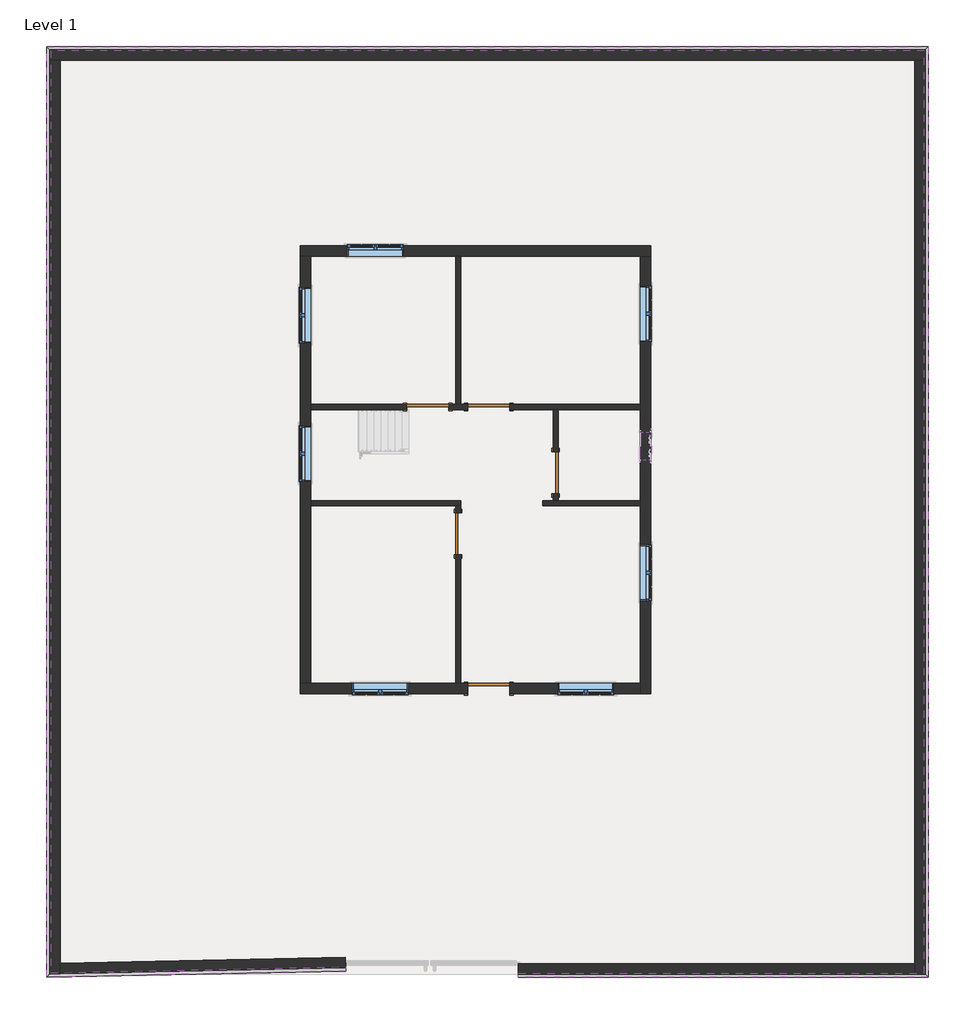
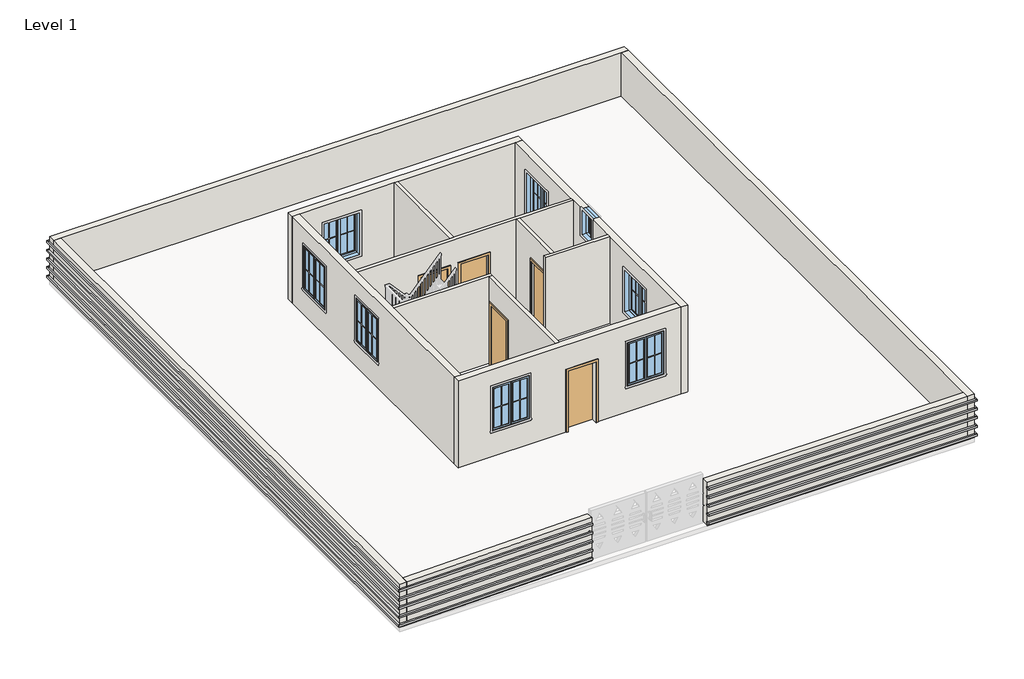
# One storey, part 1 of 2: 15 walls, 8 windows, 5 doors, 5 proxies.
"""IFC4 building model written with IfcOpenShell, lengths in millimetres."""

from ifc_helpers import new_model, si_unit, frame, origin, origin_with_axes, place, context, project, spatial, polyline, outline, extrude, faceted_brep, transform, mapped, element, save
from components import door_e5f9f3c4, door_305aa2a5, door_a90ba1ad, window_c417fced, window_8377141f

model = new_model("IFC4")

# Units and contexts
model_context = context("Model", 3, world=origin())
ifc_project = project(units=[si_unit("LENGTHUNIT", "METRE", prefix="MILLI")], contexts=[model_context])

# Site, building, storey
site = spatial("IfcSite", under=ifc_project)
building = spatial("IfcBuilding", under=site)
storey = spatial("IfcBuildingStorey", under=building, Name="Level 1", Elevation=0.0)

# Proxies
placement = place(None, origin())
element("IfcBuildingElementProxy", 1, Name="Reveal", ObjectType="Reveal", at=placement, inside=storey, context=model_context, shape_type="SweptSolid", body=[
    extrude(outline(polyline([(2255.7966432, -1211.2677992), (2257.6773598, -1303.3235895), (-4248.7407144, -1436.2508925), (-4156.6657144, -1342.2755699), (2255.7966432, -1211.2677992)])), frame((0.0, 0.0, 76.2), z_axis=(0.0, 0.0, 1.0), x_axis=(1.0, 0.0, 0.0)), (0.0, 0.0, 1.0), 67.7333333),
    extrude(outline(polyline([(14842.5342856, -1350.8294573), (14934.6092856, -1442.9044573), (6016.0342856, -1442.9044573), (6016.0342856, -1350.8294573), (14842.5342856, -1350.8294573)])), frame((0.0, 0.0, 76.2), z_axis=(0.0, 0.0, 1.0), x_axis=(1.0, 0.0, 0.0)), (0.0, 0.0, 1.0), 67.7333333),
    extrude(outline(polyline([(14842.5342856, 18715.1705427), (14934.6092856, 18807.2455427), (14934.6092856, -1442.9044573), (14842.5342856, -1350.8294573), (14842.5342856, 18715.1705427)])), frame((0.0, 0.0, 76.2), z_axis=(0.0, 0.0, 1.0), x_axis=(1.0, 0.0, 0.0)), (0.0, 0.0, 1.0), 67.7333333),
    extrude(outline(polyline([(-4156.6657144, 18715.1705427), (-4248.7407144, 18807.2455427), (14934.6092856, 18807.2455427), (14842.5342856, 18715.1705427), (-4156.6657144, 18715.1705427)])), frame((0.0, 0.0, 76.2), z_axis=(0.0, 0.0, 1.0), x_axis=(1.0, 0.0, 0.0)), (0.0, 0.0, 1.0), 67.7333333),
    extrude(outline(polyline([(-4156.6657144, -1342.2755699), (-4248.7407144, -1436.2508925), (-4248.7407144, 18807.2455427), (-4156.6657144, 18715.1705427), (-4156.6657144, -1342.2755699)])), frame((0.0, 0.0, 76.2), z_axis=(0.0, 0.0, 1.0), x_axis=(1.0, 0.0, 0.0)), (0.0, 0.0, 1.0), 67.7333333),
])
element("IfcBuildingElementProxy", 2, Name="Reveal", ObjectType="Reveal", at=placement, inside=storey, context=model_context, shape_type="SweptSolid", body=[
    extrude(outline(polyline([(2255.7966432, -1211.2677992), (2257.6773598, -1303.3235895), (-4248.7407144, -1436.2508925), (-4156.6657144, -1342.2755699), (2255.7966432, -1211.2677992)])), frame((0.0, 0.0, 381.0), z_axis=(0.0, 0.0, 1.0), x_axis=(1.0, 0.0, 0.0)), (0.0, 0.0, 1.0), 67.7333333),
    extrude(outline(polyline([(14842.5342856, -1350.8294573), (14934.6092856, -1442.9044573), (6016.0342856, -1442.9044573), (6016.0342856, -1350.8294573), (14842.5342856, -1350.8294573)])), frame((0.0, 0.0, 381.0), z_axis=(0.0, 0.0, 1.0), x_axis=(1.0, 0.0, 0.0)), (0.0, 0.0, 1.0), 67.7333333),
    extrude(outline(polyline([(14842.5342856, 18715.1705427), (14934.6092856, 18807.2455427), (14934.6092856, -1442.9044573), (14842.5342856, -1350.8294573), (14842.5342856, 18715.1705427)])), frame((0.0, 0.0, 381.0), z_axis=(0.0, 0.0, 1.0), x_axis=(1.0, 0.0, 0.0)), (0.0, 0.0, 1.0), 67.7333333),
    extrude(outline(polyline([(-4156.6657144, 18715.1705427), (-4248.7407144, 18807.2455427), (14934.6092856, 18807.2455427), (14842.5342856, 18715.1705427), (-4156.6657144, 18715.1705427)])), frame((0.0, 0.0, 381.0), z_axis=(0.0, 0.0, 1.0), x_axis=(1.0, 0.0, 0.0)), (0.0, 0.0, 1.0), 67.7333333),
    extrude(outline(polyline([(-4156.6657144, -1342.2755699), (-4248.7407144, -1436.2508925), (-4248.7407144, 18807.2455427), (-4156.6657144, 18715.1705427), (-4156.6657144, -1342.2755699)])), frame((0.0, 0.0, 381.0), z_axis=(0.0, 0.0, 1.0), x_axis=(1.0, 0.0, 0.0)), (0.0, 0.0, 1.0), 67.7333333),
])
element("IfcBuildingElementProxy", 3, Name="Reveal", ObjectType="Reveal", at=placement, inside=storey, context=model_context, shape_type="SweptSolid", body=[
    extrude(outline(polyline([(2255.7966432, -1211.2677992), (2257.6773598, -1303.3235895), (-4248.7407144, -1436.2508925), (-4156.6657144, -1342.2755699), (2255.7966432, -1211.2677992)])), frame((0.0, 0.0, 685.8), z_axis=(0.0, 0.0, 1.0), x_axis=(1.0, 0.0, 0.0)), (0.0, 0.0, 1.0), 67.7333333),
    extrude(outline(polyline([(14842.5342856, -1350.8294573), (14934.6092856, -1442.9044573), (6016.0342856, -1442.9044573), (6016.0342856, -1350.8294573), (14842.5342856, -1350.8294573)])), frame((0.0, 0.0, 685.8), z_axis=(0.0, 0.0, 1.0), x_axis=(1.0, 0.0, 0.0)), (0.0, 0.0, 1.0), 67.7333333),
    extrude(outline(polyline([(14842.5342856, 18715.1705427), (14934.6092856, 18807.2455427), (14934.6092856, -1442.9044573), (14842.5342856, -1350.8294573), (14842.5342856, 18715.1705427)])), frame((0.0, 0.0, 685.8), z_axis=(0.0, 0.0, 1.0), x_axis=(1.0, 0.0, 0.0)), (0.0, 0.0, 1.0), 67.7333333),
    extrude(outline(polyline([(-4156.6657144, 18715.1705427), (-4248.7407144, 18807.2455427), (14934.6092856, 18807.2455427), (14842.5342856, 18715.1705427), (-4156.6657144, 18715.1705427)])), frame((0.0, 0.0, 685.8), z_axis=(0.0, 0.0, 1.0), x_axis=(1.0, 0.0, 0.0)), (0.0, 0.0, 1.0), 67.7333333),
    extrude(outline(polyline([(-4156.6657144, -1342.2755699), (-4248.7407144, -1436.2508925), (-4248.7407144, 18807.2455427), (-4156.6657144, 18715.1705427), (-4156.6657144, -1342.2755699)])), frame((0.0, 0.0, 685.8), z_axis=(0.0, 0.0, 1.0), x_axis=(1.0, 0.0, 0.0)), (0.0, 0.0, 1.0), 67.7333333),
])
element("IfcBuildingElementProxy", 4, Name="Reveal", ObjectType="Reveal", at=placement, inside=storey, context=model_context, shape_type="SweptSolid", body=[
    extrude(outline(polyline([(2255.7966432, -1211.2677992), (2257.6773598, -1303.3235895), (-4248.7407144, -1436.2508925), (-4156.6657144, -1342.2755699), (2255.7966432, -1211.2677992)])), frame((0.0, 0.0, 990.6), z_axis=(0.0, 0.0, 1.0), x_axis=(1.0, 0.0, 0.0)), (0.0, 0.0, 1.0), 67.7333333),
    extrude(outline(polyline([(14842.5342856, -1350.8294573), (14934.6092856, -1442.9044573), (6016.0342856, -1442.9044573), (6016.0342856, -1350.8294573), (14842.5342856, -1350.8294573)])), frame((0.0, 0.0, 990.6), z_axis=(0.0, 0.0, 1.0), x_axis=(1.0, 0.0, 0.0)), (0.0, 0.0, 1.0), 67.7333333),
    extrude(outline(polyline([(14842.5342856, 18715.1705427), (14934.6092856, 18807.2455427), (14934.6092856, -1442.9044573), (14842.5342856, -1350.8294573), (14842.5342856, 18715.1705427)])), frame((0.0, 0.0, 990.6), z_axis=(0.0, 0.0, 1.0), x_axis=(1.0, 0.0, 0.0)), (0.0, 0.0, 1.0), 67.7333333),
    extrude(outline(polyline([(-4156.6657144, 18715.1705427), (-4248.7407144, 18807.2455427), (14934.6092856, 18807.2455427), (14842.5342856, 18715.1705427), (-4156.6657144, 18715.1705427)])), frame((0.0, 0.0, 990.6), z_axis=(0.0, 0.0, 1.0), x_axis=(1.0, 0.0, 0.0)), (0.0, 0.0, 1.0), 67.7333333),
    extrude(outline(polyline([(-4156.6657144, -1342.2755699), (-4248.7407144, -1436.2508925), (-4248.7407144, 18807.2455427), (-4156.6657144, 18715.1705427), (-4156.6657144, -1342.2755699)])), frame((0.0, 0.0, 990.6), z_axis=(0.0, 0.0, 1.0), x_axis=(1.0, 0.0, 0.0)), (0.0, 0.0, 1.0), 67.7333333),
])
element("IfcBuildingElementProxy", 5, Name="Reveal", ObjectType="Reveal", at=placement, inside=storey, context=model_context, shape_type="SweptSolid", body=[
    extrude(outline(polyline([(2255.7966432, -1211.2677992), (2257.6773598, -1303.3235895), (-4248.7407144, -1436.2508925), (-4156.6657144, -1342.2755699), (2255.7966432, -1211.2677992)])), frame((0.0, 0.0, 1295.4), z_axis=(0.0, 0.0, 1.0), x_axis=(1.0, 0.0, 0.0)), (0.0, 0.0, 1.0), 67.7333333),
    extrude(outline(polyline([(14842.5342856, -1350.8294573), (14934.6092856, -1442.9044573), (6016.0342856, -1442.9044573), (6016.0342856, -1350.8294573), (14842.5342856, -1350.8294573)])), frame((0.0, 0.0, 1295.4), z_axis=(0.0, 0.0, 1.0), x_axis=(1.0, 0.0, 0.0)), (0.0, 0.0, 1.0), 67.7333333),
    extrude(outline(polyline([(14842.5342856, 18715.1705427), (14934.6092856, 18807.2455427), (14934.6092856, -1442.9044573), (14842.5342856, -1350.8294573), (14842.5342856, 18715.1705427)])), frame((0.0, 0.0, 1295.4), z_axis=(0.0, 0.0, 1.0), x_axis=(1.0, 0.0, 0.0)), (0.0, 0.0, 1.0), 67.7333333),
    extrude(outline(polyline([(-4156.6657144, 18715.1705427), (-4248.7407144, 18807.2455427), (14934.6092856, 18807.2455427), (14842.5342856, 18715.1705427), (-4156.6657144, 18715.1705427)])), frame((0.0, 0.0, 1295.4), z_axis=(0.0, 0.0, 1.0), x_axis=(1.0, 0.0, 0.0)), (0.0, 0.0, 1.0), 67.7333333),
    extrude(outline(polyline([(-4156.6657144, -1342.2755699), (-4248.7407144, -1436.2508925), (-4248.7407144, 18807.2455427), (-4156.6657144, 18715.1705427), (-4156.6657144, -1342.2755699)])), frame((0.0, 0.0, 1295.4), z_axis=(0.0, 0.0, 1.0), x_axis=(1.0, 0.0, 0.0)), (0.0, 0.0, 1.0), 67.7333333),
])

# Doors
door_shape = door_e5f9f3c4(model_context)
element("IfcDoor", 6, ObjectType="Single-Flush : 36\" x 84\"", at=placement, inside=storey, context=model_context, shape_type="MappedRepresentation", body=[
    mapped(door_shape, transform((4044.95, 10966.45, 0.0), x_axis=(1.0, 0.0, 0.0), y_axis=(0.0, 1.0, 0.0), z_axis=(0.0, 0.0, 1.0))),
])
element("IfcDoor", 7, ObjectType="Single-Flush : 36\" x 84\"", at=placement, inside=storey, context=model_context, shape_type="MappedRepresentation", body=[
    mapped(door_shape, transform((4705.35, 8210.55, 0.0), x_axis=(0.0, 1.0, 0.0), y_axis=(-1.0, 0.0, 0.0), z_axis=(0.0, 0.0, 1.0))),
])
element("IfcDoor", 8, ObjectType="Single-Flush : 36\" x 84\"", at=placement, inside=storey, context=model_context, shape_type="MappedRepresentation", body=[
    mapped(door_shape, transform((6826.25, 9531.35, 0.0), x_axis=(0.0, -1.0, 0.0), y_axis=(1.0, 0.0, 0.0), z_axis=(0.0, 0.0, 1.0))),
])
door_2_shape = door_305aa2a5(model_context)
element("IfcDoor", 9, ObjectType="Single-Flush : 36\" x 84\"", at=placement, inside=storey, context=model_context, shape_type="MappedRepresentation", body=[
    mapped(door_2_shape, transform((5365.75, 10966.45, 0.0), x_axis=(-1.0, 0.0, 0.0), y_axis=(0.0, -1.0, 0.0), z_axis=(0.0, 0.0, 1.0))),
])
door_3_shape = door_a90ba1ad(model_context)
element("IfcDoor", 10, ObjectType="Single-Flush : 36\" x 84\"", at=placement, inside=storey, context=model_context, shape_type="MappedRepresentation", body=[
    mapped(door_3_shape, transform((5372.1, 4838.7, 0.0), x_axis=(-1.0, 0.0, 0.0), y_axis=(0.0, -1.0, 0.0), z_axis=(0.0, 0.0, 1.0))),
])

# Walls
element("IfcWall", 11, ObjectType="Generic - 5\"", at=placement, inside=storey, context=model_context, shape_type="SweptSolid", body=[
    extrude(outline(polyline([(4648.2, 11023.6), (4648.2, 14249.4), (4762.5, 14249.4), (4762.5, 11023.6), (4648.2, 11023.6)])), origin_with_axes(), (0.0, 0.0, 1.0), 3048.0),
])
element("IfcWall", 12, ObjectType="Generic - 5\"", at=placement, inside=storey, context=model_context, shape_type="Brep", body=[
    faceted_brep([(4502.15, 10909.3, 0.0), (4908.55, 10909.3, 0.0), (4908.55, 10909.3, 2133.6), (5822.95, 10909.3, 2133.6), (5822.95, 10909.3, 0.0), (6769.1, 10909.3, 0.0), (6883.4, 10909.3, 0.0), (8661.4, 10909.3, 0.0), (8661.4, 10909.3, 3048.0), (6883.4, 10909.3, 3048.0), (6769.1, 10909.3, 3048.0), (1498.6, 10909.3, 3048.0), (1498.6, 10909.3, 0.0), (3587.75, 10909.3, 0.0), (3587.75, 10909.3, 2133.6), (4502.15, 10909.3, 2133.6), (4908.55, 11023.6, 2133.6), (4908.55, 11023.6, 0.0), (4762.5, 11023.6, 0.0), (4648.2, 11023.6, 0.0), (4502.15, 11023.6, 0.0), (4502.15, 11023.6, 2133.6), (3587.75, 11023.6, 2133.6), (3587.75, 11023.6, 0.0), (1498.6, 11023.6, 0.0), (1498.6, 11023.6, 3048.0), (4648.2, 11023.6, 3048.0), (4762.5, 11023.6, 3048.0), (8661.4, 11023.6, 3048.0), (8661.4, 11023.6, 0.0), (5822.95, 11023.6, 0.0), (5822.95, 11023.6, 2133.6)], [[[0, 1, 2, 3, 4, 5, 6, 7, 8, 9, 10, 11, 12, 13, 14, 15]], [[16, 17, 18, 19, 20, 21, 22, 23, 24, 25, 26, 27, 28, 29, 30, 31]], [[13, 12, 24, 23]], [[30, 29, 7, 6, 5, 4]], [[20, 19, 18, 17, 1, 0]], [[11, 10, 9, 8, 28, 27, 26, 25]], [[8, 7, 29, 28]], [[12, 11, 25, 24]], [[21, 20, 0, 15]], [[22, 21, 15, 14]], [[23, 22, 14, 13]], [[2, 1, 17, 16]], [[3, 2, 16, 31]], [[4, 3, 31, 30]]]),
])
element("IfcWall", 13, ObjectType="Generic - 5\"", at=placement, inside=storey, context=model_context, shape_type="SweptSolid", body=[
    extrude(outline(polyline([(9074.15, 2133.6), (9074.15, 0.0), (8928.1, 0.0), (8928.1, 3048.0), (10909.3, 3048.0), (10909.3, 0.0), (9988.55, 0.0), (9988.55, 2133.6), (9074.15, 2133.6)])), frame((6769.1, 0.0, 0.0), z_axis=(1.0, 0.0, 0.0), x_axis=(0.0, 1.0, 0.0)), (0.0, 0.0, 1.0), 114.3),
])
element("IfcWall", 14, ObjectType="Generic - 5\"", at=placement, inside=storey, context=model_context, shape_type="Brep", body=[
    faceted_brep([(1498.6, 8813.8, 0.0), (4648.2, 8813.8, 0.0), (4762.5, 8813.8, 0.0), (4762.5, 8813.8, 3048.0), (4648.2, 8813.8, 3048.0), (1498.6, 8813.8, 3048.0), (1498.6, 8928.1, 0.0), (1498.6, 8928.1, 3048.0), (4762.5, 8928.1, 3048.0), (4762.5, 8928.1, 0.0)], [[[0, 1, 2, 3, 4, 5]], [[6, 7, 8, 9]], [[2, 1, 0, 6, 9]], [[5, 4, 3, 8, 7]], [[0, 5, 7, 6]], [[3, 2, 9, 8]]]),
])
element("IfcWall", 15, ObjectType="Generic - 5\"", at=placement, inside=storey, context=model_context, shape_type="SweptSolid", body=[
    extrude(outline(polyline([(8813.8, 0.0), (8667.75, 0.0), (8667.75, 2133.6), (7753.35, 2133.6), (7753.35, 0.0), (4953.0, 0.0), (4953.0, 3048.0), (8813.8, 3048.0), (8813.8, 0.0)])), frame((4648.2, 0.0, 0.0), z_axis=(1.0, 0.0, 0.0), x_axis=(0.0, 1.0, 0.0)), (0.0, 0.0, 1.0), 114.3),
])
element("IfcWall", 16, ObjectType="Generic - 5\"", at=placement, inside=storey, context=model_context, shape_type="Brep", body=[
    faceted_brep([(6540.5050896, 8813.8, 0.0), (8661.4, 8813.8, 0.0), (8661.4, 8813.8, 3048.0), (6540.5050896, 8813.8, 3048.0), (6540.5050896, 8928.1, 0.0), (6540.5050896, 8928.1, 3048.0), (6769.1, 8928.1, 3048.0), (6883.4, 8928.1, 3048.0), (8661.4, 8928.1, 3048.0), (8661.4, 8928.1, 0.0), (6883.4, 8928.1, 0.0), (6769.1, 8928.1, 0.0)], [[[0, 1, 2, 3]], [[4, 5, 6, 7, 8, 9, 10, 11]], [[1, 0, 4, 11, 10, 9]], [[3, 2, 8, 7, 6, 5]], [[0, 3, 5, 4]], [[2, 1, 9, 8]]]),
])
element("IfcWall", 17, ObjectType="Generic - 8\"", at=placement, inside=storey, context=model_context, shape_type="Brep", body=[
    faceted_brep([(1270.0, 14249.4, 0.0), (1498.6, 14249.4, 0.0), (4648.2, 14249.4, 0.0), (4762.5, 14249.4, 0.0), (8661.4, 14249.4, 0.0), (8890.0, 14249.4, 0.0), (8890.0, 14249.4, 3048.0), (8661.4, 14249.4, 3048.0), (4762.5, 14249.4, 3048.0), (4648.2, 14249.4, 3048.0), (1498.6, 14249.4, 3048.0), (1270.0, 14249.4, 3048.0), (3514.725, 14249.4, 2438.4), (3514.725, 14249.4, 914.4), (2295.525, 14249.4, 914.4), (2295.525, 14249.4, 2438.4), (1270.0, 14478.0, 0.0), (1270.0, 14478.0, 3048.0), (8890.0, 14478.0, 3048.0), (8890.0, 14478.0, 0.0), (3514.725, 14478.0, 2438.4), (2295.525, 14478.0, 2438.4), (2295.525, 14478.0, 914.4), (3514.725, 14478.0, 914.4)], [[[0, 1, 2, 3, 4, 5, 6, 7, 8, 9, 10, 11], [12, 13, 14, 15]], [[16, 17, 18, 19], [20, 21, 22, 23]], [[5, 4, 3, 2, 1, 0, 16, 19]], [[6, 5, 19, 18]], [[0, 11, 17, 16]], [[11, 10, 9, 8, 7, 6, 18, 17]], [[13, 12, 20, 23]], [[14, 13, 23, 22]], [[15, 14, 22, 21]], [[12, 15, 21, 20]]]),
])
element("IfcWall", 18, ObjectType="Generic - 8\"", at=placement, inside=storey, context=model_context, shape_type="Brep", body=[
    faceted_brep([(8661.4, 14249.4, 0.0), (8661.4, 11023.6, 0.0), (8661.4, 10909.3, 0.0), (8661.4, 8928.1, 0.0), (8661.4, 8813.8, 0.0), (8661.4, 4953.0, 0.0), (8661.4, 4724.4, 0.0), (8661.4, 4724.4, 3048.0), (8661.4, 4953.0, 3048.0), (8661.4, 8813.8, 3048.0), (8661.4, 8928.1, 3048.0), (8661.4, 9810.75, 3048.0), (8661.4, 9810.75, 2133.6), (8661.4, 10420.35, 2133.6), (8661.4, 10420.35, 3048.0), (8661.4, 10909.3, 3048.0), (8661.4, 11023.6, 3048.0), (8661.4, 14249.4, 3048.0), (8661.4, 12382.5, 2438.4), (8661.4, 12382.5, 914.4), (8661.4, 13601.7, 914.4), (8661.4, 13601.7, 2438.4), (8661.4, 6750.05, 2438.4), (8661.4, 6750.05, 914.4), (8661.4, 7969.25, 914.4), (8661.4, 7969.25, 2438.4), (8890.0, 4724.4, 0.0), (8890.0, 14249.4, 0.0), (8890.0, 14249.4, 3048.0), (8890.0, 10420.35, 3048.0), (8890.0, 10420.35, 2133.6), (8890.0, 9810.75, 2133.6), (8890.0, 9810.75, 3048.0), (8890.0, 4724.4, 3048.0), (8890.0, 12382.5, 914.4), (8890.0, 12382.5, 2438.4), (8890.0, 13601.7, 2438.4), (8890.0, 13601.7, 914.4), (8890.0, 6750.05, 914.4), (8890.0, 6750.05, 2438.4), (8890.0, 7969.25, 2438.4), (8890.0, 7969.25, 914.4)], [[[0, 1, 2, 3, 4, 5, 6, 7, 8, 9, 10, 11, 12, 13, 14, 15, 16, 17], [18, 19, 20, 21], [22, 23, 24, 25]], [[26, 27, 28, 29, 30, 31, 32, 33], [34, 35, 36, 37], [38, 39, 40, 41]], [[6, 5, 4, 3, 2, 1, 0, 27, 26]], [[0, 17, 28, 27]], [[7, 6, 26, 33]], [[7, 33, 32, 11, 10, 9, 8]], [[28, 17, 16, 15, 14, 29]], [[19, 18, 35, 34]], [[20, 19, 34, 37]], [[21, 20, 37, 36]], [[18, 21, 36, 35]], [[23, 22, 39, 38]], [[24, 23, 38, 41]], [[25, 24, 41, 40]], [[22, 25, 40, 39]], [[31, 12, 11, 32]], [[12, 31, 30, 13]], [[13, 30, 29, 14]]]),
])
element("IfcWall", 19, ObjectType="Generic - 8\"", at=placement, inside=storey, context=model_context, shape_type="Brep", body=[
    faceted_brep([(4914.9, 4953.0, 2133.6), (4914.9, 4953.0, 0.0), (4762.5, 4953.0, 0.0), (4648.2, 4953.0, 0.0), (1498.6, 4953.0, 0.0), (1270.0, 4953.0, 0.0), (1270.0, 4953.0, 3048.0), (1498.6, 4953.0, 3048.0), (4648.2, 4953.0, 3048.0), (4762.5, 4953.0, 3048.0), (8661.4, 4953.0, 3048.0), (8661.4, 4953.0, 0.0), (5829.3, 4953.0, 0.0), (5829.3, 4953.0, 2133.6), (6872.2875, 4953.0, 2438.4), (6872.2875, 4953.0, 914.4), (8091.4875, 4953.0, 914.4), (8091.4875, 4953.0, 2438.4), (2400.3, 4953.0, 2438.4), (2400.3, 4953.0, 914.4), (3619.5, 4953.0, 914.4), (3619.5, 4953.0, 2438.4), (1270.0, 4724.4, 0.0), (4914.9, 4724.4, 0.0), (4914.9, 4724.4, 2133.6), (5829.3, 4724.4, 2133.6), (5829.3, 4724.4, 0.0), (8661.4, 4724.4, 0.0), (8661.4, 4724.4, 3048.0), (1270.0, 4724.4, 3048.0), (6872.2875, 4724.4, 2438.4), (8091.4875, 4724.4, 2438.4), (8091.4875, 4724.4, 914.4), (6872.2875, 4724.4, 914.4), (2400.3, 4724.4, 2438.4), (3619.5, 4724.4, 2438.4), (3619.5, 4724.4, 914.4), (2400.3, 4724.4, 914.4)], [[[0, 1, 2, 3, 4, 5, 6, 7, 8, 9, 10, 11, 12, 13], [14, 15, 16, 17], [18, 19, 20, 21]], [[22, 23, 24, 25, 26, 27, 28, 29], [30, 31, 32, 33], [34, 35, 36, 37]], [[12, 11, 27, 26]], [[5, 4, 3, 2, 1, 23, 22]], [[11, 10, 28, 27]], [[6, 5, 22, 29]], [[24, 23, 1, 0]], [[25, 24, 0, 13]], [[26, 25, 13, 12]], [[10, 9, 8, 7, 6, 29, 28]], [[15, 14, 30, 33]], [[16, 15, 33, 32]], [[17, 16, 32, 31]], [[14, 17, 31, 30]], [[19, 18, 34, 37]], [[20, 19, 37, 36]], [[21, 20, 36, 35]], [[18, 21, 35, 34]]]),
])
element("IfcWall", 20, ObjectType="Generic - 8\"", at=placement, inside=storey, context=model_context, shape_type="Brep", body=[
    faceted_brep([(1498.6, 4953.0, 0.0), (1498.6, 8813.8, 0.0), (1498.6, 8928.1, 0.0), (1498.6, 10909.3, 0.0), (1498.6, 11023.6, 0.0), (1498.6, 14249.4, 0.0), (1498.6, 14249.4, 3048.0), (1498.6, 11023.6, 3048.0), (1498.6, 10909.3, 3048.0), (1498.6, 8928.1, 3048.0), (1498.6, 8813.8, 3048.0), (1498.6, 4953.0, 3048.0), (1498.6, 10560.05, 2438.4), (1498.6, 10560.05, 914.4), (1498.6, 9340.85, 914.4), (1498.6, 9340.85, 2438.4), (1498.6, 13569.95, 2438.4), (1498.6, 13569.95, 914.4), (1498.6, 12350.75, 914.4), (1498.6, 12350.75, 2438.4), (1270.0, 4953.0, 0.0), (1270.0, 4953.0, 3048.0), (1270.0, 14249.4, 3048.0), (1270.0, 14249.4, 0.0), (1270.0, 10560.05, 2438.4), (1270.0, 9340.85, 2438.4), (1270.0, 9340.85, 914.4), (1270.0, 10560.05, 914.4), (1270.0, 13569.95, 2438.4), (1270.0, 12350.75, 2438.4), (1270.0, 12350.75, 914.4), (1270.0, 13569.95, 914.4)], [[[0, 1, 2, 3, 4, 5, 6, 7, 8, 9, 10, 11], [12, 13, 14, 15], [16, 17, 18, 19]], [[20, 21, 22, 23], [24, 25, 26, 27], [28, 29, 30, 31]], [[5, 4, 3, 2, 1, 0, 20, 23]], [[6, 5, 23, 22]], [[0, 11, 21, 20]], [[11, 10, 9, 8, 7, 6, 22, 21]], [[13, 12, 24, 27]], [[14, 13, 27, 26]], [[15, 14, 26, 25]], [[12, 15, 25, 24]], [[17, 16, 28, 31]], [[18, 17, 31, 30]], [[19, 18, 30, 29]], [[16, 19, 29, 28]]]),
])
element("IfcWall", 21, ObjectType="Generic - 8\"", at=placement, inside=storey, context=model_context, shape_type="Brep", body=[
    faceted_brep([(-4182.0657144, 18511.9705427, 0.0), (-3953.4657144, 18511.9705427, 0.0), (14639.3342856, 18511.9705427, 0.0), (14867.9342856, 18511.9705427, 0.0), (14867.9342856, 18511.9705427, 76.2), (14842.5342856, 18511.9705427, 76.2), (14842.5342856, 18511.9705427, 143.9333333), (14867.9342856, 18511.9705427, 143.9333333), (14867.9342856, 18511.9705427, 381.0), (14842.5342856, 18511.9705427, 381.0), (14842.5342856, 18511.9705427, 448.7333333), (14867.9342856, 18511.9705427, 448.7333333), (14867.9342856, 18511.9705427, 685.8), (14842.5342856, 18511.9705427, 685.8), (14842.5342856, 18511.9705427, 753.5333333), (14867.9342856, 18511.9705427, 753.5333333), (14867.9342856, 18511.9705427, 990.6), (14842.5342856, 18511.9705427, 990.6), (14842.5342856, 18511.9705427, 1058.3333333), (14867.9342856, 18511.9705427, 1058.3333333), (14867.9342856, 18511.9705427, 1295.4), (14842.5342856, 18511.9705427, 1295.4), (14842.5342856, 18511.9705427, 1363.1333333), (14867.9342856, 18511.9705427, 1363.1333333), (14867.9342856, 18511.9705427, 1524.0), (14639.3342856, 18511.9705427, 1524.0), (-3953.4657144, 18511.9705427, 1524.0), (-4182.0657144, 18511.9705427, 1524.0), (-4182.0657144, 18511.9705427, 1363.1333333), (-4156.6657144, 18511.9705427, 1363.1333333), (-4156.6657144, 18511.9705427, 1295.4), (-4182.0657144, 18511.9705427, 1295.4), (-4182.0657144, 18511.9705427, 1058.3333333), (-4156.6657144, 18511.9705427, 1058.3333333), (-4156.6657144, 18511.9705427, 990.6), (-4182.0657144, 18511.9705427, 990.6), (-4182.0657144, 18511.9705427, 753.5333333), (-4156.6657144, 18511.9705427, 753.5333333), (-4156.6657144, 18511.9705427, 685.8), (-4182.0657144, 18511.9705427, 685.8), (-4182.0657144, 18511.9705427, 448.7333333), (-4156.6657144, 18511.9705427, 448.7333333), (-4156.6657144, 18511.9705427, 381.0), (-4182.0657144, 18511.9705427, 381.0), (-4182.0657144, 18511.9705427, 143.9333333), (-4156.6657144, 18511.9705427, 143.9333333), (-4156.6657144, 18511.9705427, 76.2), (-4182.0657144, 18511.9705427, 76.2), (14867.9342856, 18740.5705427, 0.0), (-4182.0657144, 18740.5705427, 0.0), (-4182.0657144, 18740.5705427, 76.2), (14867.9342856, 18740.5705427, 76.2), (-4182.0657144, 18740.5705427, 1524.0), (14867.9342856, 18740.5705427, 1524.0), (14867.9342856, 18740.5705427, 1363.1333333), (-4182.0657144, 18740.5705427, 1363.1333333), (14867.9342856, 18740.5705427, 143.9333333), (-4182.0657144, 18740.5705427, 143.9333333), (-4182.0657144, 18740.5705427, 381.0), (14867.9342856, 18740.5705427, 381.0), (14867.9342856, 18740.5705427, 448.7333333), (-4182.0657144, 18740.5705427, 448.7333333), (-4182.0657144, 18740.5705427, 685.8), (14867.9342856, 18740.5705427, 685.8), (14867.9342856, 18740.5705427, 753.5333333), (-4182.0657144, 18740.5705427, 753.5333333), (-4182.0657144, 18740.5705427, 990.6), (14867.9342856, 18740.5705427, 990.6), (14867.9342856, 18740.5705427, 1058.3333333), (-4182.0657144, 18740.5705427, 1058.3333333), (-4182.0657144, 18740.5705427, 1295.4), (14867.9342856, 18740.5705427, 1295.4), (14842.5342856, 18715.1705427, 143.9333333), (-4156.6657144, 18715.1705427, 143.9333333), (-4156.6657144, 18715.1705427, 76.2), (14842.5342856, 18715.1705427, 76.2), (14842.5342856, 18715.1705427, 448.7333333), (-4156.6657144, 18715.1705427, 448.7333333), (-4156.6657144, 18715.1705427, 381.0), (14842.5342856, 18715.1705427, 381.0), (14842.5342856, 18715.1705427, 753.5333333), (-4156.6657144, 18715.1705427, 753.5333333), (-4156.6657144, 18715.1705427, 685.8), (14842.5342856, 18715.1705427, 685.8), (14842.5342856, 18715.1705427, 1058.3333333), (-4156.6657144, 18715.1705427, 1058.3333333), (-4156.6657144, 18715.1705427, 990.6), (14842.5342856, 18715.1705427, 990.6), (14842.5342856, 18715.1705427, 1363.1333333), (-4156.6657144, 18715.1705427, 1363.1333333), (-4156.6657144, 18715.1705427, 1295.4), (14842.5342856, 18715.1705427, 1295.4)], [[[0, 1, 2, 3, 4, 5, 6, 7, 8, 9, 10, 11, 12, 13, 14, 15, 16, 17, 18, 19, 20, 21, 22, 23, 24, 25, 26, 27, 28, 29, 30, 31, 32, 33, 34, 35, 36, 37, 38, 39, 40, 41, 42, 43, 44, 45, 46, 47]], [[48, 49, 50, 51]], [[52, 53, 54, 55]], [[56, 57, 58, 59]], [[60, 61, 62, 63]], [[64, 65, 66, 67]], [[68, 69, 70, 71]], [[3, 2, 1, 0, 49, 48]], [[27, 26, 25, 24, 53, 52]], [[3, 48, 51, 4]], [[53, 24, 23, 54]], [[7, 56, 59, 8]], [[11, 60, 63, 12]], [[15, 64, 67, 16]], [[19, 68, 71, 20]], [[27, 52, 55, 28]], [[49, 0, 47, 50]], [[57, 44, 43, 58]], [[61, 40, 39, 62]], [[65, 36, 35, 66]], [[69, 32, 31, 70]], [[72, 73, 45, 44, 57, 56, 7, 6]], [[74, 75, 5, 4, 51, 50, 47, 46]], [[73, 74, 46, 45]], [[73, 72, 75, 74]], [[75, 72, 6, 5]], [[76, 77, 41, 40, 61, 60, 11, 10]], [[78, 79, 9, 8, 59, 58, 43, 42]], [[77, 78, 42, 41]], [[77, 76, 79, 78]], [[79, 76, 10, 9]], [[80, 81, 37, 36, 65, 64, 15, 14]], [[82, 83, 13, 12, 63, 62, 39, 38]], [[81, 82, 38, 37]], [[81, 80, 83, 82]], [[83, 80, 14, 13]], [[84, 85, 33, 32, 69, 68, 19, 18]], [[86, 87, 17, 16, 67, 66, 35, 34]], [[85, 86, 34, 33]], [[85, 84, 87, 86]], [[87, 84, 18, 17]], [[88, 89, 29, 28, 55, 54, 23, 22]], [[90, 91, 21, 20, 71, 70, 31, 30]], [[89, 90, 30, 29]], [[89, 88, 91, 90]], [[91, 88, 22, 21]]]),
])
element("IfcWall", 22, ObjectType="Generic - 8\"", at=placement, inside=storey, context=model_context, shape_type="Brep", body=[
    faceted_brep([(14639.3342856, 18511.9705427, 0.0), (14639.3342856, -1147.6294573, 0.0), (14639.3342856, -1376.2294573, 0.0), (14639.3342856, -1376.2294573, 76.2), (14639.3342856, -1350.8294573, 76.2), (14639.3342856, -1350.8294573, 143.9333333), (14639.3342856, -1376.2294573, 143.9333333), (14639.3342856, -1376.2294573, 381.0), (14639.3342856, -1350.8294573, 381.0), (14639.3342856, -1350.8294573, 448.7333333), (14639.3342856, -1376.2294573, 448.7333333), (14639.3342856, -1376.2294573, 685.8), (14639.3342856, -1350.8294573, 685.8), (14639.3342856, -1350.8294573, 753.5333333), (14639.3342856, -1376.2294573, 753.5333333), (14639.3342856, -1376.2294573, 990.6), (14639.3342856, -1350.8294573, 990.6), (14639.3342856, -1350.8294573, 1058.3333333), (14639.3342856, -1376.2294573, 1058.3333333), (14639.3342856, -1376.2294573, 1295.4), (14639.3342856, -1350.8294573, 1295.4), (14639.3342856, -1350.8294573, 1363.1333333), (14639.3342856, -1376.2294573, 1363.1333333), (14639.3342856, -1376.2294573, 1524.0), (14639.3342856, -1147.6294573, 1524.0), (14639.3342856, 18511.9705427, 1524.0), (14867.9342856, -1376.2294573, 0.0), (14867.9342856, 18511.9705427, 0.0), (14867.9342856, 18511.9705427, 76.2), (14867.9342856, -1376.2294573, 76.2), (14867.9342856, 18511.9705427, 1524.0), (14867.9342856, -1376.2294573, 1524.0), (14867.9342856, -1376.2294573, 1363.1333333), (14867.9342856, 18511.9705427, 1363.1333333), (14867.9342856, -1376.2294573, 143.9333333), (14867.9342856, 18511.9705427, 143.9333333), (14867.9342856, 18511.9705427, 381.0), (14867.9342856, -1376.2294573, 381.0), (14867.9342856, -1376.2294573, 448.7333333), (14867.9342856, 18511.9705427, 448.7333333), (14867.9342856, 18511.9705427, 685.8), (14867.9342856, -1376.2294573, 685.8), (14867.9342856, -1376.2294573, 753.5333333), (14867.9342856, 18511.9705427, 753.5333333), (14867.9342856, 18511.9705427, 990.6), (14867.9342856, -1376.2294573, 990.6), (14867.9342856, -1376.2294573, 1058.3333333), (14867.9342856, 18511.9705427, 1058.3333333), (14867.9342856, 18511.9705427, 1295.4), (14867.9342856, -1376.2294573, 1295.4), (14842.5342856, 18511.9705427, 1363.1333333), (14842.5342856, 18511.9705427, 1295.4), (14842.5342856, 18511.9705427, 1058.3333333), (14842.5342856, 18511.9705427, 990.6), (14842.5342856, 18511.9705427, 753.5333333), (14842.5342856, 18511.9705427, 685.8), (14842.5342856, 18511.9705427, 448.7333333), (14842.5342856, 18511.9705427, 381.0), (14842.5342856, 18511.9705427, 143.9333333), (14842.5342856, 18511.9705427, 76.2), (14842.5342856, -1350.8294573, 143.9333333), (14842.5342856, -1350.8294573, 76.2), (14842.5342856, -1350.8294573, 448.7333333), (14842.5342856, -1350.8294573, 381.0), (14842.5342856, -1350.8294573, 753.5333333), (14842.5342856, -1350.8294573, 685.8), (14842.5342856, -1350.8294573, 1058.3333333), (14842.5342856, -1350.8294573, 990.6), (14842.5342856, -1350.8294573, 1363.1333333), (14842.5342856, -1350.8294573, 1295.4)], [[[0, 1, 2, 3, 4, 5, 6, 7, 8, 9, 10, 11, 12, 13, 14, 15, 16, 17, 18, 19, 20, 21, 22, 23, 24, 25]], [[26, 27, 28, 29]], [[30, 31, 32, 33]], [[34, 35, 36, 37]], [[38, 39, 40, 41]], [[42, 43, 44, 45]], [[46, 47, 48, 49]], [[2, 1, 0, 27, 26]], [[25, 24, 23, 31, 30]], [[0, 25, 30, 33, 50, 51, 48, 47, 52, 53, 44, 43, 54, 55, 40, 39, 56, 57, 36, 35, 58, 59, 28, 27]], [[2, 26, 29, 3]], [[31, 23, 22, 32]], [[6, 34, 37, 7]], [[10, 38, 41, 11]], [[14, 42, 45, 15]], [[18, 46, 49, 19]], [[5, 60, 58, 35, 34, 6]], [[59, 61, 4, 3, 29, 28]], [[60, 61, 59, 58]], [[61, 60, 5, 4]], [[9, 62, 56, 39, 38, 10]], [[57, 63, 8, 7, 37, 36]], [[62, 63, 57, 56]], [[63, 62, 9, 8]], [[13, 64, 54, 43, 42, 14]], [[55, 65, 12, 11, 41, 40]], [[64, 65, 55, 54]], [[65, 64, 13, 12]], [[17, 66, 52, 47, 46, 18]], [[53, 67, 16, 15, 45, 44]], [[66, 67, 53, 52]], [[67, 66, 17, 16]], [[21, 68, 50, 33, 32, 22]], [[51, 69, 20, 19, 49, 48]], [[68, 69, 51, 50]], [[69, 68, 21, 20]]]),
])
element("IfcWall", 23, ObjectType="Generic - 8\"", at=placement, inside=storey, context=model_context, shape_type="SweptSolid", body=[
    extrude(outline(polyline([(-1147.6294573, 1524.0), (-1147.6294573, 0.0), (-1376.2294573, 0.0), (-1376.2294573, 76.2), (-1350.8294573, 76.2), (-1350.8294573, 143.9333333), (-1376.2294573, 143.9333333), (-1376.2294573, 381.0), (-1350.8294573, 381.0), (-1350.8294573, 448.7333333), (-1376.2294573, 448.7333333), (-1376.2294573, 685.8), (-1350.8294573, 685.8), (-1350.8294573, 753.5333333), (-1376.2294573, 753.5333333), (-1376.2294573, 990.6), (-1350.8294573, 990.6), (-1350.8294573, 1058.3333333), (-1376.2294573, 1058.3333333), (-1376.2294573, 1295.4), (-1350.8294573, 1295.4), (-1350.8294573, 1363.1333333), (-1376.2294573, 1363.1333333), (-1376.2294573, 1524.0), (-1147.6294573, 1524.0)])), frame((6016.0342856, 0.0, 0.0), z_axis=(1.0, 0.0, 0.0), x_axis=(0.0, 1.0, 0.0)), (0.0, 0.0, 1.0), 8623.3),
])
element("IfcWall", 24, ObjectType="Generic - 8\"", at=placement, inside=storey, context=model_context, shape_type="Brep", body=[
    faceted_brep([(-3953.4657144, -1363.5294573, 0.0), (-3953.4657144, -1134.8817543, 0.0), (-3953.4657144, 18511.9705427, 0.0), (-3953.4657144, 18511.9705427, 1524.0), (-3953.4657144, -1134.8817543, 1524.0), (-3953.4657144, -1363.5294573, 1524.0), (-3953.4657144, -1363.5294573, 1363.1333333), (-3953.4657144, -1338.124157, 1363.1333333), (-3953.4657144, -1338.124157, 1295.4), (-3953.4657144, -1363.5294573, 1295.4), (-3953.4657144, -1363.5294573, 1058.3333333), (-3953.4657144, -1338.124157, 1058.3333333), (-3953.4657144, -1338.124157, 990.6), (-3953.4657144, -1363.5294573, 990.6), (-3953.4657144, -1363.5294573, 753.5333333), (-3953.4657144, -1338.124157, 753.5333333), (-3953.4657144, -1338.124157, 685.8), (-3953.4657144, -1363.5294573, 685.8), (-3953.4657144, -1363.5294573, 448.7333333), (-3953.4657144, -1338.124157, 448.7333333), (-3953.4657144, -1338.124157, 381.0), (-3953.4657144, -1363.5294573, 381.0), (-3953.4657144, -1363.5294573, 143.9333333), (-3953.4657144, -1338.124157, 143.9333333), (-3953.4657144, -1338.124157, 76.2), (-3953.4657144, -1363.5294573, 76.2), (-4182.0657144, 18511.9705427, 0.0), (-4182.0657144, -1368.1997968, 0.0), (-4182.0657144, -1368.1997968, 76.2), (-4182.0657144, 18511.9705427, 76.2), (-4182.0657144, -1368.1997968, 1524.0), (-4182.0657144, 18511.9705427, 1524.0), (-4182.0657144, 18511.9705427, 1363.1333333), (-4182.0657144, -1368.1997968, 1363.1333333), (-4182.0657144, 18511.9705427, 143.9333333), (-4182.0657144, -1368.1997968, 143.9333333), (-4182.0657144, -1368.1997968, 381.0), (-4182.0657144, 18511.9705427, 381.0), (-4182.0657144, 18511.9705427, 448.7333333), (-4182.0657144, -1368.1997968, 448.7333333), (-4182.0657144, -1368.1997968, 685.8), (-4182.0657144, 18511.9705427, 685.8), (-4182.0657144, 18511.9705427, 753.5333333), (-4182.0657144, -1368.1997968, 753.5333333), (-4182.0657144, -1368.1997968, 990.6), (-4182.0657144, 18511.9705427, 990.6), (-4182.0657144, 18511.9705427, 1058.3333333), (-4182.0657144, -1368.1997968, 1058.3333333), (-4182.0657144, -1368.1997968, 1295.4), (-4182.0657144, 18511.9705427, 1295.4), (-4156.6657144, 18511.9705427, 76.2), (-4156.6657144, 18511.9705427, 143.9333333), (-4156.6657144, 18511.9705427, 381.0), (-4156.6657144, 18511.9705427, 448.7333333), (-4156.6657144, 18511.9705427, 685.8), (-4156.6657144, 18511.9705427, 753.5333333), (-4156.6657144, 18511.9705427, 990.6), (-4156.6657144, 18511.9705427, 1058.3333333), (-4156.6657144, 18511.9705427, 1295.4), (-4156.6657144, 18511.9705427, 1363.1333333), (-4156.6657144, -1342.2755699, 143.9333333), (-4156.6657144, -1342.2755699, 76.2), (-4156.6657144, -1342.2755699, 448.7333333), (-4156.6657144, -1342.2755699, 381.0), (-4156.6657144, -1342.2755699, 753.5333333), (-4156.6657144, -1342.2755699, 685.8), (-4156.6657144, -1342.2755699, 1058.3333333), (-4156.6657144, -1342.2755699, 990.6), (-4156.6657144, -1342.2755699, 1363.1333333), (-4156.6657144, -1342.2755699, 1295.4)], [[[0, 1, 2, 3, 4, 5, 6, 7, 8, 9, 10, 11, 12, 13, 14, 15, 16, 17, 18, 19, 20, 21, 22, 23, 24, 25]], [[26, 27, 28, 29]], [[30, 31, 32, 33]], [[34, 35, 36, 37]], [[38, 39, 40, 41]], [[42, 43, 44, 45]], [[46, 47, 48, 49]], [[2, 1, 0, 27, 26]], [[5, 4, 3, 31, 30]], [[3, 2, 26, 29, 50, 51, 34, 37, 52, 53, 38, 41, 54, 55, 42, 45, 56, 57, 46, 49, 58, 59, 32, 31]], [[5, 30, 33, 6]], [[27, 0, 25, 28]], [[35, 22, 21, 36]], [[39, 18, 17, 40]], [[43, 14, 13, 44]], [[47, 10, 9, 48]], [[51, 60, 23, 22, 35, 34]], [[24, 61, 50, 29, 28, 25]], [[60, 61, 24, 23]], [[61, 60, 51, 50]], [[53, 62, 19, 18, 39, 38]], [[20, 63, 52, 37, 36, 21]], [[62, 63, 20, 19]], [[63, 62, 53, 52]], [[55, 64, 15, 14, 43, 42]], [[16, 65, 54, 41, 40, 17]], [[64, 65, 16, 15]], [[65, 64, 55, 54]], [[57, 66, 11, 10, 47, 46]], [[12, 67, 56, 45, 44, 13]], [[66, 67, 12, 11]], [[67, 66, 57, 56]], [[59, 68, 7, 6, 33, 32]], [[8, 69, 58, 49, 48, 9]], [[68, 69, 8, 7]], [[69, 68, 59, 58]]]),
])
element("IfcWall", 25, ObjectType="Generic - 8\"", at=placement, inside=storey, context=model_context, shape_type="Brep", body=[
    faceted_brep([(2251.6460964, -1008.110193, 0.0), (-3953.4657144, -1134.8817543, 0.0), (-3953.4657144, -1134.8817543, 1524.0), (2251.6460964, -1008.110193, 1524.0), (-3953.4657144, -1363.5294573, 0.0), (2256.3154616, -1236.6625, 0.0), (2256.3154616, -1236.6625, 76.2), (-3953.4657144, -1363.5294573, 76.2), (2256.3154616, -1236.6625, 1524.0), (-3953.4657144, -1363.5294573, 1524.0), (-3953.4657144, -1363.5294573, 1363.1333333), (2256.3154616, -1236.6625, 1363.1333333), (-3953.4657144, -1363.5294573, 143.9333333), (2256.3154616, -1236.6625, 143.9333333), (2256.3154616, -1236.6625, 381.0), (-3953.4657144, -1363.5294573, 381.0), (-3953.4657144, -1363.5294573, 448.7333333), (2256.3154616, -1236.6625, 448.7333333), (2256.3154616, -1236.6625, 685.8), (-3953.4657144, -1363.5294573, 685.8), (-3953.4657144, -1363.5294573, 753.5333333), (2256.3154616, -1236.6625, 753.5333333), (2256.3154616, -1236.6625, 990.6), (-3953.4657144, -1363.5294573, 990.6), (-3953.4657144, -1363.5294573, 1058.3333333), (2256.3154616, -1236.6625, 1058.3333333), (2256.3154616, -1236.6625, 1295.4), (-3953.4657144, -1363.5294573, 1295.4), (2255.7966432, -1211.2677992, 1363.1333333), (2255.7966432, -1211.2677992, 1295.4), (2255.7966432, -1211.2677992, 1058.3333333), (2255.7966432, -1211.2677992, 990.6), (2255.7966432, -1211.2677992, 753.5333333), (2255.7966432, -1211.2677992, 685.8), (2255.7966432, -1211.2677992, 448.7333333), (2255.7966432, -1211.2677992, 381.0), (2255.7966432, -1211.2677992, 143.9333333), (2255.7966432, -1211.2677992, 76.2), (-3953.4657144, -1338.124157, 76.2), (-3953.4657144, -1338.124157, 143.9333333), (-3953.4657144, -1338.124157, 381.0), (-3953.4657144, -1338.124157, 448.7333333), (-3953.4657144, -1338.124157, 685.8), (-3953.4657144, -1338.124157, 753.5333333), (-3953.4657144, -1338.124157, 990.6), (-3953.4657144, -1338.124157, 1058.3333333), (-3953.4657144, -1338.124157, 1295.4), (-3953.4657144, -1338.124157, 1363.1333333)], [[[0, 1, 2, 3]], [[4, 5, 6, 7]], [[8, 9, 10, 11]], [[12, 13, 14, 15]], [[16, 17, 18, 19]], [[20, 21, 22, 23]], [[24, 25, 26, 27]], [[1, 0, 5, 4]], [[3, 2, 9, 8]], [[0, 3, 8, 11, 28, 29, 26, 25, 30, 31, 22, 21, 32, 33, 18, 17, 34, 35, 14, 13, 36, 37, 6, 5]], [[2, 1, 4, 7, 38, 39, 12, 15, 40, 41, 16, 19, 42, 43, 20, 23, 44, 45, 24, 27, 46, 47, 10, 9]], [[39, 36, 13, 12]], [[37, 38, 7, 6]], [[36, 39, 38, 37]], [[41, 34, 17, 16]], [[35, 40, 15, 14]], [[34, 41, 40, 35]], [[43, 32, 21, 20]], [[33, 42, 19, 18]], [[32, 43, 42, 33]], [[45, 30, 25, 24]], [[31, 44, 23, 22]], [[30, 45, 44, 31]], [[47, 28, 11, 10]], [[29, 46, 27, 26]], [[28, 47, 46, 29]]]),
])

# Windows
window_shape = window_c417fced(model_context)
element("IfcWindow", 26, ObjectType="Window-Casement-Double : 24\" x 36\"", at=placement, inside=storey, context=model_context, shape_type="MappedRepresentation", body=[
    mapped(window_shape, transform((8775.7, 10115.55, 1219.2), x_axis=(0.0, -1.0, 0.0), y_axis=(1.0, 0.0, 0.0), z_axis=(0.0, 0.0, 1.0))),
])
window_2_shape = window_8377141f(model_context)
element("IfcWindow", 27, ObjectType="Window-Casement-Double : 48\" x 60\"", at=placement, inside=storey, context=model_context, shape_type="MappedRepresentation", body=[
    mapped(window_2_shape, transform((2905.125, 14363.7, 0.0), x_axis=(1.0, 0.0, 0.0), y_axis=(0.0, 1.0, 0.0), z_axis=(0.0, 0.0, 1.0))),
])
element("IfcWindow", 28, ObjectType="Window-Casement-Double : 48\" x 60\"", at=placement, inside=storey, context=model_context, shape_type="MappedRepresentation", body=[
    mapped(window_2_shape, transform((8775.7, 12992.1, 0.0), x_axis=(0.0, -1.0, 0.0), y_axis=(1.0, 0.0, 0.0), z_axis=(0.0, 0.0, 1.0))),
])
element("IfcWindow", 29, ObjectType="Window-Casement-Double : 48\" x 60\"", at=placement, inside=storey, context=model_context, shape_type="MappedRepresentation", body=[
    mapped(window_2_shape, transform((8775.7, 7359.65, 0.0), x_axis=(0.0, -1.0, 0.0), y_axis=(1.0, 0.0, 0.0), z_axis=(0.0, 0.0, 1.0))),
])
element("IfcWindow", 30, ObjectType="Window-Casement-Double : 48\" x 60\"", at=placement, inside=storey, context=model_context, shape_type="MappedRepresentation", body=[
    mapped(window_2_shape, transform((7481.8875, 4838.7, 0.0), x_axis=(-1.0, 0.0, 0.0), y_axis=(0.0, -1.0, 0.0), z_axis=(0.0, 0.0, 1.0))),
])
element("IfcWindow", 31, ObjectType="Window-Casement-Double : 48\" x 60\"", at=placement, inside=storey, context=model_context, shape_type="MappedRepresentation", body=[
    mapped(window_2_shape, transform((3009.9, 4838.7, 0.0), x_axis=(-1.0, 0.0, 0.0), y_axis=(0.0, -1.0, 0.0), z_axis=(0.0, 0.0, 1.0))),
])
element("IfcWindow", 32, ObjectType="Window-Casement-Double : 48\" x 60\"", at=placement, inside=storey, context=model_context, shape_type="MappedRepresentation", body=[
    mapped(window_2_shape, transform((1384.3, 9950.45, 0.0), x_axis=(0.0, 1.0, 0.0), y_axis=(-1.0, 0.0, 0.0), z_axis=(0.0, 0.0, 1.0))),
])
element("IfcWindow", 33, ObjectType="Window-Casement-Double : 48\" x 60\"", at=placement, inside=storey, context=model_context, shape_type="MappedRepresentation", body=[
    mapped(window_2_shape, transform((1384.3, 12960.35, 0.0), x_axis=(0.0, 1.0, 0.0), y_axis=(-1.0, 0.0, 0.0), z_axis=(0.0, 0.0, 1.0))),
])

save(model, "model.ifc")

# Revit data of these elements
# Type "Single-Flush : 36\" x 84\""
#   Type Mark = "1"
#   Construction Type Id = "MDOOR"
#   Assembly Code = "C1020"
#   Analytic Construction = "Metal"
#   Thickness = 0' - 2"
#   Heat Transfer Coefficient (U) = 0.651978 BTU/(h·ft²·°F)
#   Height = 7' - 0"
#   Trim Projection Ext = 0' - 1"
#   Trim Projection Int = 0' - 1"
#   Trim Width = 0' - 3"
#   Width = 3' - 0"
#   Define Thermal Properties by = 1
#   Define Thermal Properties by = 1
#   Door Material = Door - Panel
#   Frame Material = Door - Frame
#   Visual Light Transmittance = 0
#   Solar Heat Gain Coefficient = 0
#   Function = (empty or 0)
#   Wall Closure = (empty or 0)
# Type "Generic - 5\""
#   Assembly Code = "B2010"
#   Layers, outside or top first: 0' - 4 1/2" no material (function 1)
# Type "Generic - 8\""
#   Assembly Code = "B2010"
#   Layers, outside or top first: 0' - 9" "Parking Stripe" (function 1)
# Type "Window-Casement-Double : 24\" x 36\""
#   Type Mark = "14"
#   Fire Rating = "0.5h"
#   Assembly Code = "B2020100"
#   Analytic Construction = "Double glazing - domestic"
#   Frame Extension [instance default] = 0' - 0 1/4"
#   Window Inset [instance default] = 0' - 0"
#   Wall Thickness [instance default] = 0' - 6"
#   Interior Wall Closure [instance default] = 0' - 2 1/4"
#   Half Width = 1' - 0"
#   Visual Light Transmittance = 0.81
#   Thermal Resistance (R) = 1.8146 (h·ft²·°F)/BTU
#   Solar Heat Gain Coefficient = 0.76
#   Rough Width = 2' - 0 1/2"
#   Rough Height = 3' - 0 1/2"
#   Height = 3' - 0"
#   Heat Transfer Coefficient (U) = 0.5511 BTU/(h·ft²·°F)
#   Exterior Wall Closure [instance default] = 0' - 1 1/4"
#   Extension Jamb [instance default] = 0' - 2 1/4"
#   Default Sill Height = 3' - 0"
#   Width = 2' - 0"
#   Define Thermal Properties by = 0
#   Muntin Visibility = yes
#   Interior Trim Visibility [instance default] = yes
#   Exterior Trim Visibility [instance default] = yes
#   Extension Jamb Visibility [instance default] = yes
#   Interior Trim Material = Wood - Stained
#   Muntin Pattern = Muntin Pattern_2x2 : Muntin Pattern_2x2
#   Interior Trim = Trim-Window-Interior-Flat : Picture Frame
#   Interior Frame Material = Wood - Stained
#   Glass Panel Material = Glass
#   Exterior Trim Material = Clad - White
#   Exterior Trim = Trim-Window-Exterior-Flat : with Sill
#   Exterior Frame Material = Clad - White
#   Wall Closure = (empty or 0)
# Type "Window-Casement-Double : 48\" x 60\""
#   Type Mark = "17"
#   Fire Rating = "0.5h"
#   Assembly Code = "B2020100"
#   Analytic Construction = "Double glazing - domestic"
#   Frame Extension [instance default] = 0' - 0 1/4"
#   Window Inset [instance default] = 0' - 0"
#   Wall Thickness [instance default] = 0' - 6"
#   Interior Wall Closure [instance default] = 0' - 2 1/4"
#   Half Width = 2' - 0"
#   Visual Light Transmittance = 0.81
#   Thermal Resistance (R) = 1.8146 (h·ft²·°F)/BTU
#   Solar Heat Gain Coefficient = 0.76
#   Rough Width = 4' - 0 1/2"
#   Rough Height = 5' - 0 1/2"
#   Height = 5' - 0"
#   Heat Transfer Coefficient (U) = 0.5511 BTU/(h·ft²·°F)
#   Exterior Wall Closure [instance default] = 0' - 1 1/4"
#   Extension Jamb [instance default] = 0' - 2 1/4"
#   Default Sill Height = 3' - 0"
#   Width = 4' - 0"
#   Define Thermal Properties by = 0
#   Muntin Visibility = yes
#   Interior Trim Visibility [instance default] = yes
#   Exterior Trim Visibility [instance default] = yes
#   Extension Jamb Visibility [instance default] = yes
#   Interior Trim Material = Wood - Stained
#   Muntin Pattern = Muntin Pattern_2x2 : Muntin Pattern_2x2
#   Interior Trim = Trim-Window-Interior-Flat : Picture Frame
#   Interior Frame Material = Wood - Stained
#   Glass Panel Material = Glass
#   Exterior Trim Material = Clad - White
#   Exterior Trim = Trim-Window-Exterior-Flat : with Sill
#   Exterior Frame Material = Clad - White
#   Wall Closure = (empty or 0)
# Elements 6, 7, 8, 9, 10 (IfcDoor, "Single-Flush : 36\" x 84\"")
#   Phase Created = New Construction
#   Materials on its faces: "Door - Frame", "Door - Panel"
# Elements 11, 12, 13, 14, 15, 16 (IfcWall, "Generic - 5\"")
#   Top Offset = 0' - 0"
#   Base Offset = 0' - 0"
#   wall height = 10' - 0"
#   Phase Created = New Construction
#   Base Constraint = Level 1
#   Top Constraint = Level 2
#   Materials on its faces: "Default Wall"
# Elements 17, 18, 19, 20 (IfcWall, "Generic - 8\"")
#   Top Offset = 0' - 0"
#   Base Offset = 0' - 0"
#   Unconnected Height = 10' - 0"
#   wall height = 10' - 0"
#   Phase Created = New Construction
#   Base Constraint = Level 1
#   Materials on its faces: "Parking Stripe", "Wood Planks"
# Elements 21, 22, 23, 24, 25 (IfcWall, "Generic - 8\"")
#   Top Offset = 0' - 0"
#   Base Offset = 0' - 0"
#   Unconnected Height = 5' - 0"
#   wall height = 5' - 0"
#   Phase Created = New Construction
#   Base Constraint = Level 1
#   Materials on its faces: "Parking Stripe", "Textile - Linen, Smooth", "Wood - Stained"
# Element 26 (IfcWindow, "Window-Casement-Double : 24\" x 36\"")
#   Mark = "8"
#   Window Inset = 0' - 0"
#   Interior Wall Closure = 0' - 2 1/4"
#   Frame Extension = 0' - 0 1/4"
#   Exterior Wall Closure = 0' - 1 1/4"
#   Interior Trim Visibility = yes
#   Exterior Trim Visibility = yes
#   Phase Created = New Construction
#   Materials on its faces: "Wood - Stained", "Glass", "Clad - White"
# Element 27 (IfcWindow, "Window-Casement-Double : 48\" x 60\"")
#   Mark = "1"
#   Window Inset = 0' - 0"
#   Interior Wall Closure = 0' - 2 1/4"
#   Frame Extension = 0' - 0 1/4"
#   Exterior Wall Closure = 0' - 1 1/4"
#   Interior Trim Visibility = yes
#   Exterior Trim Visibility = yes
#   Phase Created = New Construction
#   Materials on its faces: "Wood - Stained", "Glass", "Clad - White"
# Element 28 (IfcWindow, "Window-Casement-Double : 48\" x 60\"")
#   Mark = "2"
#   Window Inset = 0' - 0"
#   Interior Wall Closure = 0' - 2 1/4"
#   Frame Extension = 0' - 0 1/4"
#   Exterior Wall Closure = 0' - 1 1/4"
#   Interior Trim Visibility = yes
#   Exterior Trim Visibility = yes
#   Phase Created = New Construction
#   Materials on its faces: "Wood - Stained", "Glass", "Clad - White"
# Element 29 (IfcWindow, "Window-Casement-Double : 48\" x 60\"")
#   Mark = "3"
#   Window Inset = 0' - 0"
#   Interior Wall Closure = 0' - 2 1/4"
#   Frame Extension = 0' - 0 1/4"
#   Exterior Wall Closure = 0' - 1 1/4"
#   Interior Trim Visibility = yes
#   Exterior Trim Visibility = yes
#   Phase Created = New Construction
#   Materials on its faces: "Wood - Stained", "Glass", "Clad - White"
# Element 30 (IfcWindow, "Window-Casement-Double : 48\" x 60\"")
#   Mark = "4"
#   Window Inset = 0' - 0"
#   Interior Wall Closure = 0' - 2 1/4"
#   Frame Extension = 0' - 0 1/4"
#   Exterior Wall Closure = 0' - 1 1/4"
#   Interior Trim Visibility = yes
#   Exterior Trim Visibility = yes
#   Phase Created = New Construction
#   Materials on its faces: "Wood - Stained", "Glass", "Clad - White"
# Element 31 (IfcWindow, "Window-Casement-Double : 48\" x 60\"")
#   Mark = "5"
#   Window Inset = 0' - 0"
#   Interior Wall Closure = 0' - 2 1/4"
#   Frame Extension = 0' - 0 1/4"
#   Exterior Wall Closure = 0' - 1 1/4"
#   Interior Trim Visibility = yes
#   Exterior Trim Visibility = yes
#   Phase Created = New Construction
#   Materials on its faces: "Wood - Stained", "Glass", "Clad - White"
# Element 32 (IfcWindow, "Window-Casement-Double : 48\" x 60\"")
#   Mark = "6"
#   Window Inset = 0' - 0"
#   Interior Wall Closure = 0' - 2 1/4"
#   Frame Extension = 0' - 0 1/4"
#   Exterior Wall Closure = 0' - 1 1/4"
#   Interior Trim Visibility = yes
#   Exterior Trim Visibility = yes
#   Phase Created = New Construction
#   Materials on its faces: "Wood - Stained", "Glass", "Clad - White"
# Element 33 (IfcWindow, "Window-Casement-Double : 48\" x 60\"")
#   Mark = "7"
#   Window Inset = 0' - 0"
#   Interior Wall Closure = 0' - 2 1/4"
#   Frame Extension = 0' - 0 1/4"
#   Exterior Wall Closure = 0' - 1 1/4"
#   Interior Trim Visibility = yes
#   Exterior Trim Visibility = yes
#   Phase Created = New Construction
#   Materials on its faces: "Wood - Stained", "Glass", "Clad - White"
# Materials
#   "Door - Panel": class "Wood", colour RGB 210 159 95, transparency 0, Cost = 0
#   "Door - Frame": colour RGB 118 70 51, transparency 0, Cost = 0
#   "Parking Stripe": class "Paint", colour RGB 250 250 91, transparency 0, Cost = 0
#   "Wood - Stained": class "Wood", colour RGB 224 178 126, transparency 0, Cost = 0
#   "Glass": class "Glass", colour RGB 0 128 192, transparency 0.75, Description = "Soda Lime Glass", Cost = 0
#   "Clad - White": class "Wood", colour RGB 242 242 238, transparency 0, Cost = 0
#   "Default Wall": colour RGB 128 128 128, transparency 0, Cost = 0
#   "Wood Planks": class "Wood", colour RGB 193 160 115, transparency 0, Description = "Physical material.", Cost = 0
#   "Textile - Linen, Smooth": colour RGB 249 239 230, transparency 0
